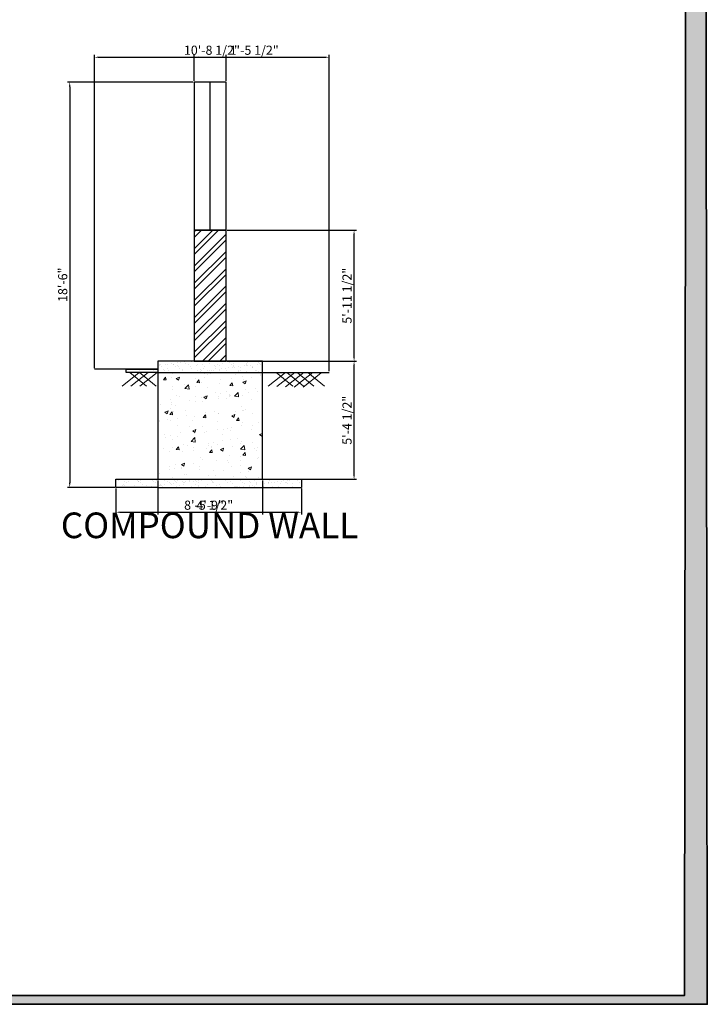
# Model space of a CAD drawing. Units: inches. Extents: x 1804 to 3296, y 909 to 2477.
# Tile 24 of 31: x 2920 to 3296, y 909 to 1449. Entities that reach past the tile are written whole.
import ezdxf

# ---------------------------------------------------------------- set-up
doc = ezdxf.new("R2010")
doc.units = ezdxf.units.IN
for name, color, linetype, lineweight in [('A-ANNO-DIMS', 2, 'Continuous', 18), ('A-ANNO-TTLB', 156, 'Continuous', 35), ('A-DETL', 7, 'Continuous', 30), ('A-DETL-PATT', 8, 'Continuous', 13), ('A-WALL-PATT', 10, 'Continuous', 13), ('C-GRAD-PATT', 8, 'Continuous', 13), ('TEXT', 190, 'Continuous', 18)]:
    doc.layers.add(name, color=color, linetype=linetype, lineweight=lineweight)
doc.styles.get("Standard").update_dxf_attribs({"font": 'arial.ttf'})
doc.dimstyles.new('ISO-25', dxfattribs={"dimtxt": 5, "dimasz": 2.5, "dimexe": 1.25, "dimexo": 0.625, "dimtad": 1, "dimdec": 0, "dimlunit": 4, "dimtxsty": 'Standard', "dimcen": 2.5, "dimadec": 0, "dimazin": 0, "dimtfac": 1, "dimtdec": 0, "dimtmove": 0, "dimatfit": 3, "dimfxl": 1, "dimarcsym": 0})

# ---------------------------------------------------------------- blocks, each defined once
blk = doc.blocks.new('*D94')
at = {"layer": 'A-ANNO-DIMS', "color": 0, "lineweight": -2, "transparency": 16777216}
for p, q in [((2972.46, 1191.87), (2972.46, 1177.65)), ((3074, 1191.87), (3074, 1177.65)), ((2974.96, 1178.9), (3071.5, 1178.9))]:
    blk.add_line(p, q, dxfattribs=at)
at = {"layer": 'A-ANNO-DIMS', "color": 0, "lineweight": 100, "transparency": 16777216}
for points in [[(2974.96, 1179.31), (2974.96, 1178.48), (2972.46, 1178.9)], [(3071.5, 1179.31), (3071.5, 1178.48), (3074, 1178.9)]]:
    blk.add_solid(points, dxfattribs=at)
at = {"layer": 'Defpoints', "color": 0, "lineweight": 100, "transparency": 16777216}
for p in [(2972.46, 1192.5), (3074, 1192.5), (3074, 1178.9)]:
    blk.add_point(p, dxfattribs=at)
at = {"layer": 'A-ANNO-DIMS', "color": 0, "transparency": 16777216, "insert": (3023.23, 1182.11), "char_height": 5, "attachment_point": 5}
blk.add_mtext('8\'-5 1/2"', dxfattribs=at)
blk = doc.blocks.new('*D95')
at = {"layer": 'A-ANNO-DIMS', "color": 0, "lineweight": -2, "transparency": 16777216}
for p, q in [((3014.75, 1414.4), (2945.94, 1414.4)), ((2947.19, 1411.9), (2947.19, 1195)), ((2971.84, 1192.5), (2945.94, 1192.5))]:
    blk.add_line(p, q, dxfattribs=at)
at = {"layer": 'A-ANNO-DIMS', "color": 0, "lineweight": 100, "transparency": 16777216}
for points in [[(2946.78, 1411.9), (2947.61, 1411.9), (2947.19, 1414.4)], [(2946.78, 1195), (2947.61, 1195), (2947.19, 1192.5)]]:
    blk.add_solid(points, dxfattribs=at)
at = {"layer": 'Defpoints', "color": 0, "lineweight": 100, "transparency": 16777216}
for p in [(3015.37, 1414.4), (2947.19, 1192.5), (2972.46, 1192.5)]:
    blk.add_point(p, dxfattribs=at)
at = {"layer": 'A-ANNO-DIMS', "color": 0, "transparency": 16777216, "insert": (2944.01, 1303.45), "char_height": 5, "attachment_point": 5, "rotation": 90}
blk.add_mtext('18\'-6"', dxfattribs=at)
blk = doc.blocks.new('*D96')
at = {"layer": 'A-ANNO-DIMS', "color": 0, "lineweight": -2, "transparency": 16777216}
for p, q in [((3015.37, 1415.02), (3015.37, 1429.25)), ((3032.82, 1415.02), (3032.82, 1429.25)), ((3017.87, 1428), (3030.32, 1428)), ((3032.82, 1428), (3061.04, 1428))]:
    blk.add_line(p, q, dxfattribs=at)
at = {"layer": 'A-ANNO-DIMS', "color": 0, "lineweight": 100, "transparency": 16777216}
for points in [[(3017.87, 1428.42), (3017.87, 1427.58), (3015.37, 1428)], [(3030.32, 1428.42), (3030.32, 1427.58), (3032.82, 1428)]]:
    blk.add_solid(points, dxfattribs=at)
at = {"layer": 'Defpoints', "color": 0, "lineweight": 100, "transparency": 16777216}
for p in [(3032.82, 1428), (3015.37, 1414.4), (3032.82, 1414.4)]:
    blk.add_point(p, dxfattribs=at)
at = {"layer": 'A-ANNO-DIMS', "color": 0, "transparency": 16777216, "insert": (3048.18, 1431.21), "char_height": 5, "attachment_point": 5}
blk.add_mtext('1\'-5 1/2"', dxfattribs=at)
blk = doc.blocks.new('*D97')
at = {"layer": 'A-ANNO-DIMS', "color": 0, "lineweight": -2, "transparency": 16777216}
for p, q in [((2995.47, 1196.29), (2995.47, 1177.65)), ((3052.66, 1196.29), (3052.66, 1177.65)), ((2997.97, 1178.9), (3050.16, 1178.9))]:
    blk.add_line(p, q, dxfattribs=at)
at = {"layer": 'A-ANNO-DIMS', "color": 0, "lineweight": 100, "transparency": 16777216}
for points in [[(2997.97, 1179.31), (2997.97, 1178.48), (2995.47, 1178.9)], [(3050.16, 1179.31), (3050.16, 1178.48), (3052.66, 1178.9)]]:
    blk.add_solid(points, dxfattribs=at)
at = {"layer": 'Defpoints', "color": 0, "lineweight": 100, "transparency": 16777216}
for p in [(2995.47, 1196.92), (3052.66, 1196.92), (3052.66, 1178.9)]:
    blk.add_point(p, dxfattribs=at)
at = {"layer": 'A-ANNO-DIMS', "color": 0, "transparency": 16777216, "insert": (3024.06, 1182.07), "char_height": 5, "attachment_point": 5}
blk.add_mtext('4\'-9"', dxfattribs=at)
blk = doc.blocks.new('*D98')
at = {"layer": 'A-ANNO-DIMS', "color": 0, "lineweight": -2, "transparency": 16777216}
for p, q in [((3053.28, 1261.58), (3104.08, 1261.58)), ((3102.83, 1199.42), (3102.83, 1259.08)), ((3053.28, 1196.92), (3104.08, 1196.92))]:
    blk.add_line(p, q, dxfattribs=at)
at = {"layer": 'A-ANNO-DIMS', "color": 0, "lineweight": 100, "transparency": 16777216}
for points in [[(3102.41, 1259.08), (3103.24, 1259.08), (3102.83, 1261.58)], [(3102.41, 1199.42), (3103.24, 1199.42), (3102.83, 1196.92)]]:
    blk.add_solid(points, dxfattribs=at)
at = {"layer": 'Defpoints', "color": 0, "lineweight": 100, "transparency": 16777216}
for p in [(3052.66, 1261.58), (3102.83, 1261.58), (3052.66, 1196.92)]:
    blk.add_point(p, dxfattribs=at)
at = {"layer": 'A-ANNO-DIMS', "color": 0, "transparency": 16777216, "insert": (3099.62, 1229.25), "char_height": 5, "attachment_point": 5, "rotation": 90}
blk.add_mtext('5\'-4 1/2"', dxfattribs=at)
blk = doc.blocks.new('*D99')
at = {"layer": 'A-ANNO-DIMS', "color": 0, "lineweight": -2, "transparency": 16777216}
for p, q in [((3033.45, 1333.28), (3104.08, 1333.28)), ((3102.83, 1264.08), (3102.83, 1330.78)), ((3033.45, 1261.58), (3104.08, 1261.58))]:
    blk.add_line(p, q, dxfattribs=at)
at = {"layer": 'A-ANNO-DIMS', "color": 0, "lineweight": 100, "transparency": 16777216}
for points in [[(3102.41, 1330.78), (3103.24, 1330.78), (3102.83, 1333.28)], [(3102.41, 1264.08), (3103.24, 1264.08), (3102.83, 1261.58)]]:
    blk.add_solid(points, dxfattribs=at)
at = {"layer": 'Defpoints', "color": 0, "lineweight": 100, "transparency": 16777216}
for p in [(3032.82, 1333.28), (3102.83, 1333.28), (3032.82, 1261.58)]:
    blk.add_point(p, dxfattribs=at)
at = {"layer": 'A-ANNO-DIMS', "color": 0, "transparency": 16777216, "insert": (3099.62, 1297.43), "char_height": 5, "attachment_point": 5, "rotation": 90}
blk.add_mtext('5\'-11 1/2"', dxfattribs=at)
blk = doc.blocks.new('*D100')
at = {"layer": 'A-ANNO-DIMS', "color": 0, "lineweight": -2, "transparency": 16777216}
for p, q in [((2960.79, 1257.86), (2960.79, 1429.25)), ((3089.23, 1256.09), (3089.23, 1429.25)), ((2963.29, 1428), (3086.73, 1428))]:
    blk.add_line(p, q, dxfattribs=at)
at = {"layer": 'A-ANNO-DIMS', "color": 0, "lineweight": 100, "transparency": 16777216}
for points in [[(2963.29, 1428.42), (2963.29, 1427.58), (2960.79, 1428)], [(3086.73, 1428.42), (3086.73, 1427.58), (3089.23, 1428)]]:
    blk.add_solid(points, dxfattribs=at)
at = {"layer": 'Defpoints', "color": 0, "lineweight": 100, "transparency": 16777216}
for p in [(3089.23, 1428), (2960.79, 1257.24), (3089.23, 1255.47)]:
    blk.add_point(p, dxfattribs=at)
at = {"layer": 'A-ANNO-DIMS', "color": 0, "transparency": 16777216, "insert": (3025.01, 1431.21), "char_height": 5, "attachment_point": 5}
blk.add_mtext('10\'-8 1/2"', dxfattribs=at)

msp = doc.modelspace()

# ---------------------------------------------------------------- hatches: boundary and pattern name
at = {"layer": 'A-ANNO-TTLB'}
h = msp.add_hatch(color=256, dxfattribs=at)
h.dxf.hatch_style = 1
h.paths.add_polyline_path([(3294.53, 2476.54), (1803.79, 2476.54), (1805.43, 909.47), (3296.17, 909.47)])
h.paths.add_polyline_path([(1811, 914.33), (1812.79, 2467.54), (3285.53, 2467.54), (3283.74, 914.33)], flags=16)
h.paths.add_polyline_path([(1925.58, 1062.77), (1925.58, 1138.07), (1925.58, 1539.88), (1925.58, 1793.38), (1925.58, 1830.04), (2325.54, 1830.04), (2325.54, 1793.38), (2325.54, 1586.42), (2325.54, 1138.07), (2325.54, 1062.77)], flags=0)
h.paths.add_polyline_path([(1997.22, 1029.4), (2008.85, 1037.96), (2008.85, 1020.84)], flags=0)
h.paths.add_polyline_path([(1934.58, 1138.07), (1934.58, 1147.07), (2078.77, 1147.07), (2078.77, 1138.07), (2060.94, 1138.07)], flags=0)
h.paths.add_polyline_path([(1944.35, 1138.07), (1944.35, 1147.07), (2056.05, 1147.07), (2056.05, 1138.07)], flags=0)
h.paths.add_polyline_path([(2222.24, 1037.96), (2233.87, 1029.4), (2222.24, 1020.84)], flags=0)
h.paths.add_polyline_path([(2061.94, 1139.07), (2061.94, 1146.07), (2077.77, 1146.07), (2077.77, 1139.07)], flags=0)
h.paths.add_polyline_path([(2149.58, 1138.07), (2149.58, 1269.44), (2158.58, 1269.44), (2158.58, 1326.69), (2149.58, 1326.69), (2149.58, 1340.94), (2139.6, 1340.94), (2139.6, 1434.25), (2149.58, 1434.25), (2149.58, 1447.36), (2158.58, 1447.36), (2158.58, 1423.87), (2158.58, 1408.06), (2198.46, 1408.06), (2198.46, 1412.56), (2282.65, 1412.56), (2282.65, 1465.94), (2316.54, 1465.94), (2316.54, 1590.92), (2192.86, 1590.92), (2192.86, 1595.3), (2291.17, 1595.3), (2291.17, 1590.92), (2316.54, 1590.92), (2316.54, 1784.38), (2300.24, 1784.38), (2300.24, 1757.47), (2268, 1757.47), (2268, 1681.04), (2180.87, 1681.04), (2180.87, 1757.47), (2148.63, 1757.47), (2148.63, 1784.38), (2119.08, 1784.38), (2119.08, 1585.58), (2114.58, 1585.58), (2114.58, 1784.38), (2064.11, 1784.38), (2046.28, 1784.38), (2046.28, 1760.38), (1958.58, 1760.38), (1958.58, 1664.38), (1934.58, 1664.38), (1934.58, 1784.38), (1934.58, 1793.38), (2046.28, 1793.38), (2064.11, 1793.38), (2119.08, 1793.38), (2230.78, 1793.38), (2230.78, 1784.38), (2268, 1784.38), (2300.24, 1784.38), (2316.54, 1784.38), (2316.54, 1590.92), (2316.54, 1373.73), (2316.54, 1138.07)], flags=0)
h.paths.add_polyline_path([(2209.19, 1166.63), (2209.19, 1175.63), (2158.58, 1175.63), (2209.19, 1223.63), (2209.19, 1231.63), (2183.88, 1231.63), (2183.88, 1301.66), (2242.59, 1301.66), (2242.59, 1326.69), (2316.54, 1326.69), (2272.59, 1271.63), (2272.59, 1223.63), (2316.54, 1175.63), (2272.59, 1175.63), (2272.59, 1166.63)], flags=0)
h.paths.add_polyline_path([(1947.77, 1345.22), (1947.77, 1457.48), (1991.2, 1457.48), (1991.2, 1451.7), (1991.2, 1352.18), (1991.2, 1345.22)], flags=0)
h.paths.add_polyline_path([(2209.19, 1271.63), (2262.59, 1271.63), (2262.59, 1311.85), (2272.59, 1301.66), (2272.59, 1271.63), (2269.92, 1269.63), (2270.59, 1269.63), (2270.59, 1225.63), (2211.19, 1225.63), (2211.19, 1269.63), (2211.86, 1269.63)], flags=0)
h.paths.add_polyline_path([(2000.34, 1378.21), (2000.34, 1429.71), (2025.22, 1429.71), (2025.22, 1378.21)], flags=0)
h.paths.add_polyline_path([(2001.34, 1379.21), (2001.34, 1428.71), (2024.22, 1428.71), (2024.22, 1379.21)], flags=0)
h.paths.add_polyline_path([(2012.34, 1390.21), (2012.34, 1417.71), (2013.22, 1417.71), (2013.22, 1390.21)], flags=0)
h.paths.add_polyline_path([(2237.56, 1331.19), (2237.56, 1340.18), (2238.62, 1340.18), (2238.62, 1386.84), (2241.04, 1386.84), (2242.06, 1386.84), (2242.06, 1408.06), (2316.54, 1331.19)], flags=0)
h.paths.add_polyline_path([(1953.73, 1464.35), (1953.73, 1498.59), (1981.74, 1498.59), (1981.74, 1464.35)], flags=0)
h.paths.add_polyline_path([(1987.63, 1462.08), (1987.63, 1500.95), (2104.07, 1500.95), (2104.07, 1462.08), (2099.27, 1462.08), (1993.6, 1462.08)], flags=0)
h.paths.add_polyline_path([(1956.06, 1481.47, -1), (1979.41, 1481.47, -1)], flags=0)
edge = h.paths.add_edge_path(flags=0)
edge.add_ellipse((2299.53, 1438.37), major_axis=(0.31, 21.36), ratio=0.670333, start_angle=0, end_angle=360)
h.paths.add_polyline_path([(2297.39, 1438.37, -1), (2301.67, 1438.37, -1)], flags=0)
h.paths.add_polyline_path([(2591.54, 1163.23), (2591.54, 1179.38), (2591.54, 1379.68), (2591.54, 1395.84), (2734.5, 1395.84), (2734.5, 1379.68), (2734.5, 1179.38), (2734.5, 1163.23)], flags=0)
h.paths.add_polyline_path([(2592.54, 1164.23), (2592.54, 1166.23), (2733.5, 1166.23), (2733.5, 1164.23)], flags=0)
h.paths.add_polyline_path([(2592.54, 1180.38), (2592.54, 1378.68), (2733.5, 1378.68), (2733.5, 1180.38)], flags=0)
h.paths.add_polyline_path([(2593.54, 1181.38), (2593.54, 1377.68), (2732.5, 1377.68), (2732.5, 1181.38)], flags=0)
h.paths.add_polyline_path([(2594.54, 1182.38), (2594.54, 1376.68), (2731.5, 1376.68), (2731.5, 1182.38)], flags=0)
h.paths.add_polyline_path([(1936.95, 1697.46), (1936.95, 1736.46), (1955.41, 1736.46), (1955.41, 1697.46)], flags=0)
h.paths.add_polyline_path([(1938.48, 1718.36), (1938.48, 1734.92), (1953.65, 1734.92), (1953.65, 1718.36)], flags=0)
h.paths.add_polyline_path([(1944.75, 1726.64, -1), (1947.37, 1726.64, -1)], flags=0)
h.paths.add_polyline_path([(2592.54, 1394.84), (2733.5, 1394.84), (2733.5, 1392.84), (2592.54, 1392.84)], flags=0)
h.paths.add_polyline_path([(1976.61, 1762.5), (1976.61, 1781.44), (2012.79, 1781.44), (2012.79, 1762.5)], flags=0)
h.paths.add_polyline_path([(1979.57, 1771.97, -1), (1991.39, 1771.97, -1)], flags=0)
h.paths.add_polyline_path([(1995.36, 1771.97, -1), (2007.18, 1771.97, -1)], flags=0)
h.paths.add_polyline_path([(2251.51, 1744.53), (2268, 1730.05), (2251.51, 1730.05)], flags=0)
h.paths.add_polyline_path([(2047.28, 1785.38), (2047.28, 1792.38), (2063.11, 1792.38), (2063.11, 1785.38)], flags=0)
h.paths.add_polyline_path([(2155.08, 1770.92, -1), (2174.42, 1770.92, -1)], flags=0)
h.paths.add_polyline_path([(2188.59, 1758.27), (2188.59, 1772.81), (2222.3, 1772.81), (2222.3, 1758.27)], flags=0)
h.paths.add_polyline_path([(2223.97, 1758.27), (2223.97, 1772.81), (2257.68, 1772.81), (2257.68, 1758.27)], flags=0)
h.paths.add_polyline_path([(2274.45, 1770.92, -1), (2293.8, 1770.92, -1)], flags=0)
h.paths.add_polyline_path([(2591.54, 1582.09), (2591.54, 1782.39), (2734.5, 1782.39), (2734.5, 1582.09)], flags=0)
h.paths.add_polyline_path([(2592.54, 1583.09), (2592.54, 1781.39), (2733.5, 1781.39), (2733.5, 1583.09)], flags=0)
h.paths.add_polyline_path([(2593.54, 1584.09), (2593.54, 1780.39), (2732.5, 1780.39), (2732.5, 1584.09)], flags=0)
h.paths.add_polyline_path([(2594.54, 1585.09), (2594.54, 1779.39), (2731.5, 1779.39), (2731.5, 1585.09)], flags=0)
h.paths.add_polyline_path([(1922.17, 1978.79), (1922.17, 2295.08), (1922.17, 2296.08), (2115.67, 2296.08), (2115.67, 2384.31), (2115.67, 2385.31), (2322.12, 2385.31), (2323.12, 2385.31), (2323.12, 1979.79), (2323.12, 1978.79), (1923.17, 1978.79)], flags=0)
h.paths.add_polyline_path([(1922.17, 1978.79), (1922.17, 2051.31), (1922.17, 2214.86), (1922.17, 2296.08), (2115.67, 2296.08), (2115.67, 2385.31), (2323.12, 2385.31), (2323.12, 2280.42), (2323.12, 1978.79), (2115.67, 1978.79)], flags=0)
h.paths.add_polyline_path([(1923.17, 1979.79), (1923.17, 2050.31), (2115.67, 2050.31), (2115.67, 2051.31), (1923.17, 2051.31), (1923.17, 2213.86), (1923.17, 2214.86), (1923.17, 2295.08), (1990.02, 2295.08), (1990.02, 2214.86), (1991.02, 2214.86), (1991.02, 2295.08), (2115.67, 2295.08), (2115.67, 1979.79), (2116.67, 1979.79), (2116.67, 2304.18), (2116.67, 2384.31), (2322.12, 2384.31), (2322.12, 2280.42), (2322.12, 1979.79), (2115.67, 1979.79)], flags=0)
h.paths.add_polyline_path([(2972.46, 1192.5), (2972.46, 1196.92), (2995.47, 1196.92), (2995.47, 1255.47), (2995.09, 1255.47), (2987.42, 1249.39), (2980.08, 1255.47), (2978.05, 1255.47), (2978.05, 1257.24), (2995.47, 1257.24), (2995.47, 1261.58), (3015.37, 1261.58), (3015.37, 1333.28), (3015.37, 1414.4), (3032.82, 1414.4), (3032.82, 1333.28), (3032.82, 1261.58), (3052.66, 1261.58), (3052.66, 1255.47), (3079.86, 1255.47), (3078.72, 1254.57), (3081.47, 1252.29), (3078.56, 1249.99), (3075.81, 1252.26), (3072.57, 1249.69), (3070.36, 1251.52), (3067.67, 1249.39), (3060.34, 1255.47), (3052.66, 1255.47), (3052.66, 1196.92), (3054.58, 1196.92), (3074, 1196.92), (3074, 1192.5), (3052.66, 1192.5), (2995.47, 1192.5)], flags=0)
h.paths.add_polyline_path([(2490.75, 1979.27), (2490.75, 1980.27), (2596.87, 1980.27), (2596.87, 2051.8), (2596.87, 2052.8), (2596.87, 2216.35), (2596.87, 2297.57), (2717.32, 2297.57), (2710.57, 2305.62), (2724.07, 2305.62), (2717.32, 2297.57), (2782.37, 2297.57), (2782.37, 2395.8), (3006.82, 2395.8), (3006.82, 1981.27), (3093.73, 1981.27), (3093.73, 1980.27), (3047.51, 1980.27), (3046.37, 1979.37), (3049.11, 1977.1), (3046.2, 1974.79), (3043.46, 1977.07), (3040.21, 1974.49), (3038, 1976.32), (3035.32, 1974.2), (3027.98, 1980.27), (2871.83, 1980.27), (2871.83, 1981.27), (2791.37, 1981.27), (2791.37, 2050.8), (2597.87, 2050.8), (2597.87, 1980.27), (2597.87, 1979.27), (2546.27, 1979.27), (2545.12, 1978.37), (2547.87, 1976.1), (2544.96, 1973.79), (2542.22, 1976.07), (2538.97, 1973.49), (2536.76, 1975.32), (2534.07, 1973.2), (2526.74, 1979.27)], flags=0)
h.paths.add_polyline_path([(2597.87, 2051.8), (2606.87, 2051.8), (2606.87, 2258.39), (2597.87, 2258.39), (2597.87, 2296.57), (2606.87, 2296.57), (2606.87, 2262.39), (2782.37, 2262.39), (2782.37, 2296.57), (2790.37, 2296.57), (2790.37, 2262.39), (2791.37, 2262.39), (2791.37, 2305.67), (2791.37, 2385.8), (2996.82, 2385.8), (2996.82, 2339.85), (3006.82, 2339.85), (3006.82, 2250.12), (2997.82, 2250.12), (2997.82, 1981.27), (2996.82, 1981.27), (2872.83, 1981.27), (2872.83, 1991.8), (2871.83, 1991.8), (2871.83, 2050.8), (2790.37, 2050.8), (2597.87, 2050.8)], flags=0)
h.paths.add_polyline_path([(2179.93, 2153.92), (2179.93, 2353.97), (2259.98, 2353.97), (2259.98, 2153.92)], flags=0)
h.paths.add_polyline_path([(2180.93, 2154.92), (2180.93, 2352.97), (2258.98, 2352.97), (2258.98, 2154.92)], flags=0)
h.paths.add_polyline_path([(2960.87, 1608.49), (2960.87, 1753.62), (3070.9, 1753.62), (3070.9, 1608.49)], flags=0)
h.paths.add_polyline_path([(2961.87, 1609.49), (2961.87, 1752.62), (3069.9, 1752.62), (3069.9, 1609.49)], flags=0)
h.paths.add_polyline_path([(2962.87, 1610.49), (2962.87, 1751.62), (3068.9, 1751.62), (3068.9, 1610.49)], flags=0)
h.paths.add_polyline_path([(2963.87, 1611.49), (2963.87, 1750.62), (3067.9, 1750.62), (3067.9, 1611.49)], flags=0)
h.paths.add_polyline_path([(2782.37, 2051.8), (2782.37, 2216.32), (2791.37, 2216.32), (2791.37, 2051.8), (2872.83, 2051.8), (2872.83, 2068.56), (2884.67, 2068.56), (2884.67, 2085.33), (2896.51, 2085.33), (2896.51, 2102.09), (2908.36, 2102.09), (2908.36, 2118.85), (2920.2, 2118.85), (2920.2, 2135.62), (2932.05, 2135.62), (2932.05, 2145.3), (2925.08, 2145.3), (2925.08, 2203.2), (2996.82, 2203.2), (2996.82, 2145.3), (2953.82, 2145.3), (2872.83, 2051.8), (2790.37, 2051.8)], flags=0)
h.paths.add_polyline_path([(2717.32, 2238.65), (2710.57, 2246.7), (2724.07, 2246.7)], flags=0)
h.paths.add_polyline_path([(2003.09, 1122.79), (2017.16, 1122.79), (2017.16, 1138.74), (2003.09, 1138.74)], flags=8)
h.paths.add_polyline_path([(2174.76, 1792.72), (2188.83, 1792.72), (2188.83, 1808.66), (2174.76, 1808.66)], flags=8)
h.paths.add_polyline_path([(1987.95, 1792.51), (2002.02, 1792.51), (2002.02, 1808.45), (1987.95, 1808.45)], flags=8)
h.paths.add_polyline_path([(2148.79, 1289.26), (2160.46, 1289.26), (2160.46, 1305.2), (2148.79, 1305.2)], flags=8)
h.paths.add_polyline_path([(2115.36, 1133.57), (2127.04, 1133.57), (2127.04, 1149.51), (2115.36, 1149.51)], flags=8)
h.paths.add_polyline_path([(2237.58, 1421.48), (2249.25, 1421.48), (2249.25, 1437.43), (2237.58, 1437.43)], flags=8)
h.paths.add_polyline_path([(2134.99, 1584.32), (2146.66, 1584.32), (2146.66, 1600.26), (2134.99, 1600.26)], flags=8)
h.paths.add_polyline_path([(2101.95, 1557.31), (2113.62, 1557.31), (2113.62, 1573.25), (2101.95, 1573.25)], flags=8)
h.paths.add_polyline_path([(2937.85, 1156.77), (3120.41, 1156.77), (3120.41, 1185.72), (2937.85, 1185.72)], flags=8)
h.paths.add_polyline_path([(2980.71, 1786.71), (3050.06, 1786.71), (3050.06, 1802.66), (2980.71, 1802.66)], flags=8)
h.paths.add_polyline_path([(2869.28, 1661.96), (2938.62, 1661.96), (2938.62, 1690.8), (2869.28, 1690.8)], flags=8)
h.paths.add_polyline_path([(3092.27, 1674.86), (3161.62, 1674.86), (3161.62, 1690.8), (3092.27, 1690.8)], flags=8)
h.paths.add_polyline_path([(2980.71, 1674.86), (3050.06, 1674.86), (3050.06, 1690.8), (2980.71, 1690.8)], flags=8)
h.paths.add_polyline_path([(2649.07, 1678.23), (2674.53, 1678.23), (2674.53, 1714.76), (2649.07, 1714.76)], flags=8)
h.paths.add_polyline_path([(2530.84, 1981.63), (2549.13, 1981.63), (2549.13, 1997.57), (2530.84, 1997.57)], flags=8)
h.paths.add_polyline_path([(3031.29, 1981.77), (3049.58, 1981.77), (3049.58, 1997.71), (3031.29, 1997.71)], flags=8)
h.paths.add_polyline_path([(2715.38, 1911.9), (2851.54, 1911.9), (2851.54, 1940.85), (2715.38, 1940.85)], flags=8)
h.paths.add_polyline_path([(2015.23, 1927.36), (2205.42, 1927.36), (2205.42, 1956.3), (2015.23, 1956.3)], flags=8)
h.paths.add_polyline_path([(2671.84, 2057.84), (2702.75, 2057.84), (2702.75, 2073.79), (2671.84, 2073.79)], flags=8)
h.paths.add_polyline_path([(2678.5, 2316.52), (2765.26, 2316.52), (2765.26, 2332.46), (2678.5, 2332.46)], flags=8)
h.paths.add_polyline_path([(2678.48, 2271.96), (2736.41, 2271.96), (2736.41, 2287.9), (2678.48, 2287.9)], flags=8)
h.paths.add_polyline_path([(2019.2, 972.79), (2243.21, 972.79), (2243.21, 1001.74), (2019.2, 1001.74)], flags=8)
h.paths.add_polyline_path([(2097.06, 1021.56), (2132.16, 1021.56), (2132.16, 1037.51), (2097.06, 1037.51)], flags=8)
h.paths.add_polyline_path([(2182.47, 1360.48), (2207.35, 1360.48), (2207.35, 1376.42), (2182.47, 1376.42)], flags=8)
h.paths.add_polyline_path([(2261.12, 1361.77), (2295.01, 1361.77), (2295.01, 1377.71), (2261.12, 1377.71)], flags=8)
h.paths.add_polyline_path([(2245.75, 1511.51), (2278.44, 1511.51), (2278.44, 1527.46), (2245.75, 1527.46)], flags=8)
h.paths.add_polyline_path([(1991.16, 1296.29), (2060.51, 1296.29), (2060.51, 1312.23), (1991.16, 1312.23)], flags=8)
h.paths.add_polyline_path([(2187, 1651.35), (2246.71, 1651.35), (2246.71, 1667.29), (2187, 1667.29)], flags=8)
h.paths.add_polyline_path([(1976.49, 1684.81), (2068.63, 1684.81), (2068.63, 1700.76), (1976.49, 1700.76)], flags=8)
at = {"layer": 'A-DETL-PATT'}
h = msp.add_hatch(dxfattribs=at)
h.set_pattern_fill('ANSI32', color=256, scale=0.7)
h.set_pattern_definition([(45, (64.579, 248.7134), (-4.714634, 4.714634), []), (45, (67.722, 248.7134), (-4.714634, 4.714634), [])])
h.paths.add_polyline_path([(3032.82, 1333.28), (3015.37, 1333.28), (3015.37, 1261.58), (3032.82, 1261.58)])
h = msp.add_hatch(dxfattribs=at)
h.set_pattern_fill('AR-SAND', color=256, scale=0.1)
h.set_pattern_definition([(37.5, (64.579, 248.7134), (-0.160003, 4.8941324), [0, -3.8608, 0, -4.318, 0, -4.1275]), (7.5, (64.579, 248.7134), (4.495233, 7.168251), [0, -2.0828, 0, -3.4798, 0, -1.3335]), (327.5, (61.4548, 248.7134), (7.9099237, 0.014372), [0, -1.27, 0, -4.572, 0, -5.969]), (317.5, (61.455, 248.7134), (7.635565, 2.229293), [0, -0.635, 0, -2.9972, 0, -3.429])])
h.paths.add_polyline_path([(3052.66, 1261.58), (2995.47, 1261.58), (2995.47, 1255.47), (3052.66, 1255.47)])
h.paths.add_polyline_path([(3074, 1196.92), (3052.66, 1196.92), (2995.47, 1196.92), (2972.46, 1196.92), (2972.46, 1192.5), (2995.47, 1192.5), (3052.66, 1192.5), (3074, 1192.5)])
h.paths.add_polyline_path([(2995.47, 1257.24), (2978.05, 1257.24), (2978.05, 1255.47), (2995.47, 1255.47)])
h = msp.add_hatch(dxfattribs=at)
h.set_pattern_fill('AR-SAND', color=256, scale=0.4)
h.set_pattern_definition([(37.5, (64.579, 248.713), (-0.64001, 19.57653), [0, -15.4432, 0, -17.272, 0, -16.51]), (7.5, (64.58, 248.713), (17.98093, 28.673), [0, -8.3312, 0, -13.9192, 0, -5.334]), (327.5, (52.082, 248.713), (31.639695, 0.05749), [0, -5.08, 0, -18.288, 0, -23.876]), (317.5, (52.082, 248.713), (30.54226, 8.91717), [0, -2.54, 0, -11.9888, 0, -13.716])])
h.paths.add_polyline_path([(2995.47, 1196.92), (3052.66, 1196.92), (3052.66, 1255.47), (2995.47, 1255.47)])
h = msp.add_hatch(dxfattribs=at)
h.set_pattern_fill('AR-CONC', color=256, scale=0.1)
h.set_pattern_definition([(50, (64.579, 248.713), (18.21847, -1.59391), [1.905, -20.955]), (355, (64.579, 248.713), (-3.52434, 19.10568), [1.524, -16.76406]), (100.45144, (66.097, 248.58), (14.69412, 17.51178), [1.619, -17.80902]), (46.1842, (64.58, 253.793), (27.1079, -4.20423), [2.8575, -31.4325]), (96.6356, (66.838, 253.443), (23.74041, 24.74261), [2.4285, -26.71356]), (351.1842, (64.58, 253.793), (23.74041, 24.7426), [2.286, -25.14597]), (21, (67.119, 252.523), (15.16144, -10.22652), [1.905, -20.955]), (326, (67.119, 252.523), (6.1802, 18.4188), [1.524, -16.764]), (71.45144, (68.382, 251.671), (21.34164, 8.19228), [1.619, -17.80899]), (37.5, (64.579, 248.7134), (0.30886, 8.455504), [0, -16.5608, 0, -17.018, 0, -16.8275]), (7.5, (64.579, 248.713), (6.681966, 10.018057), [0, -9.7028, 0, -16.1798, 0, -6.4135]), (327.5, (58.915, 248.7134), (13.55906, -0.572874), [0, -6.35, 0, -19.812, 0, -26.289]), (317.5, (56.375, 248.713), (14.81292, 2.54265), [0, -8.255, 0, -13.1572, 0, -18.669])])
h.paths.add_polyline_path([(2995.47, 1255.47), (2995.47, 1196.92), (3052.66, 1196.92), (3052.66, 1255.47)])
at = {"layer": 'A-WALL-PATT'}
h = msp.add_hatch(color=256, dxfattribs=at)
h.dxf.hatch_style = 1
h.paths.add_polyline_path([(2119.08, 1544.38), (1925.58, 1544.38), (1925.58, 1539.88), (2119.08, 1539.88)])
h.paths.add_polyline_path([(2119.08, 1545.58), (2114.58, 1545.58), (2114.58, 1544.38), (2119.08, 1544.38)])
h.paths.add_polyline_path([(1965.87, 1658.79), (1965.87, 1679.09), (1955.57, 1679.09), (1955.57, 1658.79)], flags=9)
h.paths.add_polyline_path([(2293.18, 1677.29), (2293.18, 1697.58), (2282.88, 1697.58), (2282.88, 1677.29)], flags=9)
h.paths.add_polyline_path([(2271.13, 1545.23), (2287.53, 1545.23), (2287.53, 1555.53), (2271.13, 1555.53)], flags=9)
h.paths.add_polyline_path([(2303.26, 1488.52), (2303.26, 1508.82), (2292.95, 1508.82), (2292.95, 1488.52)], flags=9)
h.paths.add_polyline_path([(2271.13, 1393.15), (2287.53, 1393.15), (2287.53, 1403.45), (2271.13, 1403.45)], flags=9)
h.paths.add_polyline_path([(2306.48, 1361.45), (2306.48, 1377.86), (2296.18, 1377.86), (2296.18, 1361.45)], flags=9)
h.paths.add_polyline_path([(2174.54, 1361.45), (2174.54, 1377.86), (2164.23, 1377.86), (2164.23, 1361.45)], flags=9)
h.paths.add_polyline_path([(1968.21, 1333.34), (1968.21, 1353.64), (1957.91, 1353.64), (1957.91, 1333.34)], flags=9)
h.paths.add_polyline_path([(2003.09, 1122.79), (2017.16, 1122.79), (2017.16, 1138.74), (2003.09, 1138.74)], flags=9)
h.paths.add_polyline_path([(2174.76, 1792.72), (2188.83, 1792.72), (2188.83, 1808.66), (2174.76, 1808.66)], flags=9)
h.paths.add_polyline_path([(1987.95, 1792.51), (2002.02, 1792.51), (2002.02, 1808.45), (1987.95, 1808.45)], flags=9)
h.paths.add_polyline_path([(2148.79, 1289.26), (2160.46, 1289.26), (2160.46, 1305.2), (2148.79, 1305.2)], flags=9)
h.paths.add_polyline_path([(2115.36, 1133.57), (2127.04, 1133.57), (2127.04, 1149.51), (2115.36, 1149.51)], flags=9)
h.paths.add_polyline_path([(2237.58, 1421.48), (2249.25, 1421.48), (2249.25, 1437.43), (2237.58, 1437.43)], flags=9)
h.paths.add_polyline_path([(2134.99, 1584.32), (2146.66, 1584.32), (2146.66, 1600.26), (2134.99, 1600.26)], flags=9)
h.paths.add_polyline_path([(2101.95, 1557.31), (2113.62, 1557.31), (2113.62, 1573.25), (2101.95, 1573.25)], flags=9)
h.paths.add_polyline_path([(2937.85, 1156.77), (3120.41, 1156.77), (3120.41, 1185.72), (2937.85, 1185.72)], flags=9)
h.paths.add_polyline_path([(2980.71, 1786.71), (3050.06, 1786.71), (3050.06, 1802.66), (2980.71, 1802.66)], flags=9)
h.paths.add_polyline_path([(2869.28, 1661.96), (2938.62, 1661.96), (2938.62, 1690.8), (2869.28, 1690.8)], flags=9)
h.paths.add_polyline_path([(3092.27, 1674.86), (3161.62, 1674.86), (3161.62, 1690.8), (3092.27, 1690.8)], flags=9)
h.paths.add_polyline_path([(2980.71, 1674.86), (3050.06, 1674.86), (3050.06, 1690.8), (2980.71, 1690.8)], flags=9)
h.paths.add_polyline_path([(2649.07, 1678.23), (2674.53, 1678.23), (2674.53, 1714.76), (2649.07, 1714.76)], flags=9)
h.paths.add_polyline_path([(2530.84, 1981.63), (2549.13, 1981.63), (2549.13, 1997.57), (2530.84, 1997.57)], flags=9)
h.paths.add_polyline_path([(3031.29, 1981.77), (3049.58, 1981.77), (3049.58, 1997.71), (3031.29, 1997.71)], flags=9)
h.paths.add_polyline_path([(2715.38, 1911.9), (2851.54, 1911.9), (2851.54, 1940.85), (2715.38, 1940.85)], flags=9)
h.paths.add_polyline_path([(2015.23, 1927.36), (2205.42, 1927.36), (2205.42, 1956.3), (2015.23, 1956.3)], flags=9)
h.paths.add_polyline_path([(2671.84, 2057.84), (2702.75, 2057.84), (2702.75, 2073.79), (2671.84, 2073.79)], flags=9)
h.paths.add_polyline_path([(2678.5, 2316.52), (2765.26, 2316.52), (2765.26, 2332.46), (2678.5, 2332.46)], flags=9)
h.paths.add_polyline_path([(2678.48, 2271.96), (2736.41, 2271.96), (2736.41, 2287.9), (2678.48, 2287.9)], flags=9)
h.paths.add_polyline_path([(2019.2, 972.79), (2243.21, 972.79), (2243.21, 1001.74), (2019.2, 1001.74)], flags=9)
h.paths.add_polyline_path([(2097.06, 1021.56), (2132.16, 1021.56), (2132.16, 1037.51), (2097.06, 1037.51)], flags=9)
h.paths.add_polyline_path([(2182.47, 1360.48), (2207.35, 1360.48), (2207.35, 1376.42), (2182.47, 1376.42)], flags=9)
h.paths.add_polyline_path([(2261.12, 1361.77), (2295.01, 1361.77), (2295.01, 1377.71), (2261.12, 1377.71)], flags=9)
h.paths.add_polyline_path([(2245.75, 1511.51), (2278.44, 1511.51), (2278.44, 1527.46), (2245.75, 1527.46)], flags=9)
h.paths.add_polyline_path([(1991.16, 1296.29), (2060.51, 1296.29), (2060.51, 1312.23), (1991.16, 1312.23)], flags=9)
h.paths.add_polyline_path([(2187, 1651.35), (2246.71, 1651.35), (2246.71, 1667.29), (2187, 1667.29)], flags=9)
h.paths.add_polyline_path([(1976.49, 1684.81), (2068.63, 1684.81), (2068.63, 1700.76), (1976.49, 1700.76)], flags=9)
h = msp.add_hatch(color=256, dxfattribs=at)
h.dxf.hatch_style = 1
h.paths.add_polyline_path([(2149.58, 1147.07), (2141.21, 1147.07), (2141.21, 1144.07), (2141.21, 1138.07), (2149.58, 1138.07)])
h.paths.add_polyline_path([(2101.21, 1144.07, -0.01877), (2101.32, 1147.07), (2078.77, 1147.07), (2078.77, 1138.07), (2101.21, 1138.07)])
h.paths.add_polyline_path([(2060.94, 1147.07), (2056.05, 1147.07), (2056.05, 1138.07), (2060.94, 1138.07)])
h.paths.add_polyline_path([(1944.35, 1147.07), (1934.58, 1147.07), (1934.58, 1138.07), (1944.35, 1138.07)])
h.paths.add_polyline_path([(2158.58, 1269.44), (2149.58, 1269.44), (2149.58, 1138.07), (2158.58, 1138.07)])
h.paths.add_polyline_path([(2003.09, 1122.79), (2017.16, 1122.79), (2017.16, 1138.74), (2003.09, 1138.74)], flags=9)
h.paths.add_polyline_path([(2174.76, 1792.72), (2188.83, 1792.72), (2188.83, 1808.66), (2174.76, 1808.66)], flags=9)
h.paths.add_polyline_path([(1987.95, 1792.51), (2002.02, 1792.51), (2002.02, 1808.45), (1987.95, 1808.45)], flags=9)
h.paths.add_polyline_path([(2148.79, 1289.26), (2160.46, 1289.26), (2160.46, 1305.2), (2148.79, 1305.2)], flags=9)
h.paths.add_polyline_path([(2115.36, 1133.57), (2127.04, 1133.57), (2127.04, 1149.51), (2115.36, 1149.51)], flags=9)
h.paths.add_polyline_path([(2237.58, 1421.48), (2249.25, 1421.48), (2249.25, 1437.43), (2237.58, 1437.43)], flags=9)
h.paths.add_polyline_path([(2134.99, 1584.32), (2146.66, 1584.32), (2146.66, 1600.26), (2134.99, 1600.26)], flags=9)
h.paths.add_polyline_path([(2101.95, 1557.31), (2113.62, 1557.31), (2113.62, 1573.25), (2101.95, 1573.25)], flags=9)
h.paths.add_polyline_path([(2937.85, 1156.77), (3120.41, 1156.77), (3120.41, 1185.72), (2937.85, 1185.72)], flags=9)
h.paths.add_polyline_path([(2980.71, 1786.71), (3050.06, 1786.71), (3050.06, 1802.66), (2980.71, 1802.66)], flags=9)
h.paths.add_polyline_path([(2869.28, 1661.96), (2938.62, 1661.96), (2938.62, 1690.8), (2869.28, 1690.8)], flags=9)
h.paths.add_polyline_path([(3092.27, 1674.86), (3161.62, 1674.86), (3161.62, 1690.8), (3092.27, 1690.8)], flags=9)
h.paths.add_polyline_path([(2980.71, 1674.86), (3050.06, 1674.86), (3050.06, 1690.8), (2980.71, 1690.8)], flags=9)
h.paths.add_polyline_path([(2649.07, 1678.23), (2674.53, 1678.23), (2674.53, 1714.76), (2649.07, 1714.76)], flags=9)
h.paths.add_polyline_path([(2530.84, 1981.63), (2549.13, 1981.63), (2549.13, 1997.57), (2530.84, 1997.57)], flags=9)
h.paths.add_polyline_path([(3031.29, 1981.77), (3049.58, 1981.77), (3049.58, 1997.71), (3031.29, 1997.71)], flags=9)
h.paths.add_polyline_path([(2715.38, 1911.9), (2851.54, 1911.9), (2851.54, 1940.85), (2715.38, 1940.85)], flags=9)
h.paths.add_polyline_path([(2015.23, 1927.36), (2205.42, 1927.36), (2205.42, 1956.3), (2015.23, 1956.3)], flags=9)
h.paths.add_polyline_path([(2671.84, 2057.84), (2702.75, 2057.84), (2702.75, 2073.79), (2671.84, 2073.79)], flags=9)
h.paths.add_polyline_path([(2678.5, 2316.52), (2765.26, 2316.52), (2765.26, 2332.46), (2678.5, 2332.46)], flags=9)
h.paths.add_polyline_path([(2678.48, 2271.96), (2736.41, 2271.96), (2736.41, 2287.9), (2678.48, 2287.9)], flags=9)
h.paths.add_polyline_path([(2019.2, 972.79), (2243.21, 972.79), (2243.21, 1001.74), (2019.2, 1001.74)], flags=9)
h.paths.add_polyline_path([(2097.06, 1021.56), (2132.16, 1021.56), (2132.16, 1037.51), (2097.06, 1037.51)], flags=9)
h.paths.add_polyline_path([(2182.47, 1360.48), (2207.35, 1360.48), (2207.35, 1376.42), (2182.47, 1376.42)], flags=9)
h.paths.add_polyline_path([(2261.12, 1361.77), (2295.01, 1361.77), (2295.01, 1377.71), (2261.12, 1377.71)], flags=9)
h.paths.add_polyline_path([(2245.75, 1511.51), (2278.44, 1511.51), (2278.44, 1527.46), (2245.75, 1527.46)], flags=9)
h.paths.add_polyline_path([(1991.16, 1296.29), (2060.51, 1296.29), (2060.51, 1312.23), (1991.16, 1312.23)], flags=9)
h.paths.add_polyline_path([(2187, 1651.35), (2246.71, 1651.35), (2246.71, 1667.29), (2187, 1667.29)], flags=9)
h.paths.add_polyline_path([(1976.49, 1684.81), (2068.63, 1684.81), (2068.63, 1700.76), (1976.49, 1700.76)], flags=9)
h = msp.add_hatch(color=256, dxfattribs=at)
h.dxf.hatch_style = 1
h.paths.add_polyline_path([(2158.58, 1275.49), (2155.29, 1275.49), (2149.58, 1275.49), (2149.58, 1269.44), (2158.58, 1269.44)])
h.paths.add_polyline_path([(2158.58, 1326.69), (2149.58, 1326.69), (2149.58, 1319.33), (2155.29, 1319.33), (2158.58, 1319.33)])
h.paths.add_polyline_path([(2158.58, 1402.2), (2158.58, 1423.87), (2158.58, 1447.36), (2149.58, 1447.36), (2149.58, 1423.87), (2149.58, 1340.94), (2149.58, 1326.69), (2158.58, 1326.69), (2158.58, 1354.23)])
h.paths.add_polyline_path([(1965.87, 1658.79), (1965.87, 1679.09), (1955.57, 1679.09), (1955.57, 1658.79)], flags=9)
h.paths.add_polyline_path([(2293.18, 1677.29), (2293.18, 1697.58), (2282.88, 1697.58), (2282.88, 1677.29)], flags=9)
h.paths.add_polyline_path([(2271.13, 1545.23), (2287.53, 1545.23), (2287.53, 1555.53), (2271.13, 1555.53)], flags=9)
h.paths.add_polyline_path([(2303.26, 1488.52), (2303.26, 1508.82), (2292.95, 1508.82), (2292.95, 1488.52)], flags=9)
h.paths.add_polyline_path([(2271.13, 1393.15), (2287.53, 1393.15), (2287.53, 1403.45), (2271.13, 1403.45)], flags=9)
h.paths.add_polyline_path([(2306.48, 1361.45), (2306.48, 1377.86), (2296.18, 1377.86), (2296.18, 1361.45)], flags=9)
h.paths.add_polyline_path([(2189.9, 1340.62), (2206.31, 1340.62), (2206.31, 1350.92), (2189.9, 1350.92)], flags=9)
h.paths.add_polyline_path([(2174.54, 1361.45), (2174.54, 1377.86), (2164.23, 1377.86), (2164.23, 1361.45)], flags=9)
h.paths.add_polyline_path([(2304.24, 1240.8), (2304.24, 1261.09), (2293.94, 1261.09), (2293.94, 1240.8)], flags=9)
h.paths.add_polyline_path([(2227.19, 1188.73), (2247.49, 1188.73), (2247.49, 1199.03), (2227.19, 1199.03)], flags=9)
h.paths.add_polyline_path([(2181.93, 1144.21), (2181.93, 1160.62), (2171.63, 1160.62), (2171.63, 1144.21)], flags=9)
h.paths.add_polyline_path([(1968.21, 1333.34), (1968.21, 1353.64), (1957.91, 1353.64), (1957.91, 1333.34)], flags=9)
h.paths.add_polyline_path([(2029.78, 1203.53), (2053.95, 1203.53), (2053.95, 1213.83), (2029.78, 1213.83)], flags=9)
h.paths.add_polyline_path([(2576.51, 1671.88), (2576.51, 1692.17), (2566.21, 1692.17), (2566.21, 1671.88)], flags=9)
h.paths.add_polyline_path([(2566.99, 1269.67), (2566.99, 1289.96), (2556.68, 1289.96), (2556.68, 1269.67)], flags=9)
h.paths.add_polyline_path([(2581.85, 1269.17), (2581.85, 1289.46), (2571.54, 1289.46), (2571.54, 1269.17)], flags=9)
h.paths.add_polyline_path([(2650.71, 1409.75), (2674.89, 1409.75), (2674.89, 1420.05), (2650.71, 1420.05)], flags=9)
h.paths.add_polyline_path([(2003.09, 1122.79), (2017.16, 1122.79), (2017.16, 1138.74), (2003.09, 1138.74)], flags=9)
h.paths.add_polyline_path([(2174.76, 1792.72), (2188.83, 1792.72), (2188.83, 1808.66), (2174.76, 1808.66)], flags=9)
h.paths.add_polyline_path([(1987.95, 1792.51), (2002.02, 1792.51), (2002.02, 1808.45), (1987.95, 1808.45)], flags=9)
h.paths.add_polyline_path([(2148.79, 1289.26), (2160.46, 1289.26), (2160.46, 1305.2), (2148.79, 1305.2)], flags=9)
h.paths.add_polyline_path([(2115.36, 1133.57), (2127.04, 1133.57), (2127.04, 1149.51), (2115.36, 1149.51)], flags=9)
h.paths.add_polyline_path([(2237.58, 1421.48), (2249.25, 1421.48), (2249.25, 1437.43), (2237.58, 1437.43)], flags=9)
h.paths.add_polyline_path([(2134.99, 1584.32), (2146.66, 1584.32), (2146.66, 1600.26), (2134.99, 1600.26)], flags=9)
h.paths.add_polyline_path([(2101.95, 1557.31), (2113.62, 1557.31), (2113.62, 1573.25), (2101.95, 1573.25)], flags=9)
h.paths.add_polyline_path([(2937.85, 1156.77), (3120.41, 1156.77), (3120.41, 1185.72), (2937.85, 1185.72)], flags=9)
h.paths.add_polyline_path([(2980.71, 1786.71), (3050.06, 1786.71), (3050.06, 1802.66), (2980.71, 1802.66)], flags=9)
h.paths.add_polyline_path([(2869.28, 1661.96), (2938.62, 1661.96), (2938.62, 1690.8), (2869.28, 1690.8)], flags=9)
h.paths.add_polyline_path([(3092.27, 1674.86), (3161.62, 1674.86), (3161.62, 1690.8), (3092.27, 1690.8)], flags=9)
h.paths.add_polyline_path([(2980.71, 1674.86), (3050.06, 1674.86), (3050.06, 1690.8), (2980.71, 1690.8)], flags=9)
h.paths.add_polyline_path([(2649.07, 1678.23), (2674.53, 1678.23), (2674.53, 1714.76), (2649.07, 1714.76)], flags=9)
h.paths.add_polyline_path([(2530.84, 1981.63), (2549.13, 1981.63), (2549.13, 1997.57), (2530.84, 1997.57)], flags=9)
h.paths.add_polyline_path([(3031.29, 1981.77), (3049.58, 1981.77), (3049.58, 1997.71), (3031.29, 1997.71)], flags=9)
h.paths.add_polyline_path([(2715.38, 1911.9), (2851.54, 1911.9), (2851.54, 1940.85), (2715.38, 1940.85)], flags=9)
h.paths.add_polyline_path([(2015.23, 1927.36), (2205.42, 1927.36), (2205.42, 1956.3), (2015.23, 1956.3)], flags=9)
h.paths.add_polyline_path([(2671.84, 2057.84), (2702.75, 2057.84), (2702.75, 2073.79), (2671.84, 2073.79)], flags=9)
h.paths.add_polyline_path([(2678.5, 2316.52), (2765.26, 2316.52), (2765.26, 2332.46), (2678.5, 2332.46)], flags=9)
h.paths.add_polyline_path([(2678.48, 2271.96), (2736.41, 2271.96), (2736.41, 2287.9), (2678.48, 2287.9)], flags=9)
h.paths.add_polyline_path([(2019.2, 972.79), (2243.21, 972.79), (2243.21, 1001.74), (2019.2, 1001.74)], flags=9)
h.paths.add_polyline_path([(2097.06, 1021.56), (2132.16, 1021.56), (2132.16, 1037.51), (2097.06, 1037.51)], flags=9)
h.paths.add_polyline_path([(2182.47, 1360.48), (2207.35, 1360.48), (2207.35, 1376.42), (2182.47, 1376.42)], flags=9)
h.paths.add_polyline_path([(2261.12, 1361.77), (2295.01, 1361.77), (2295.01, 1377.71), (2261.12, 1377.71)], flags=9)
h.paths.add_polyline_path([(2245.75, 1511.51), (2278.44, 1511.51), (2278.44, 1527.46), (2245.75, 1527.46)], flags=9)
h.paths.add_polyline_path([(1991.16, 1296.29), (2060.51, 1296.29), (2060.51, 1312.23), (1991.16, 1312.23)], flags=9)
h.paths.add_polyline_path([(2187, 1651.35), (2246.71, 1651.35), (2246.71, 1667.29), (2187, 1667.29)], flags=9)
h.paths.add_polyline_path([(1976.49, 1684.81), (2068.63, 1684.81), (2068.63, 1700.76), (1976.49, 1700.76)], flags=9)
at = {"layer": 'C-GRAD-PATT'}
h = msp.add_hatch(dxfattribs=at)
h.set_pattern_fill('ANSI31', color=256, scale=0.953826, angle=-6.62272, style=0)
h.paths.add_polyline_path([(2974.43, 1247.99), (2987.11, 1247.99), (2996.55, 1255.47), (2983.87, 1255.47)])
h = msp.add_hatch(dxfattribs=at)
h.set_pattern_fill('ANSI31', color=256, scale=1.053974, angle=95.36535, style=0)
h.paths.add_polyline_path([(2978.51, 1255.47), (2987.6, 1247.94), (2995.99, 1247.94), (2986.9, 1255.47)])
h = msp.add_hatch(dxfattribs=at)
h.set_pattern_fill('ANSI31', color=256, scale=0.971184, angle=-6.62272, style=0)
h.paths.add_polyline_path([(3054.66, 1247.99), (3073.69, 1247.31), (3076.67, 1247.31), (3086.11, 1254.79), (3081.35, 1255.47), (3064.1, 1255.47)])
h = msp.add_hatch(dxfattribs=at)
h.set_pattern_fill('ANSI31', color=256, scale=1.157881, angle=95.36535, style=0)
h.paths.add_polyline_path([(3058.61, 1255.47), (3067.7, 1247.94), (3088.45, 1247.94), (3079.36, 1255.47)])

# ---------------------------------------------------------------- linework, layer by layer
at = {"layer": 'A-ANNO-TTLB'}
for points in [[(1803.79, 2476.54), (3294.53, 2476.54), (3296.17, 909.47), (1805.43, 909.47)], [(1812.79, 2467.54), (3285.53, 2467.54), (3283.74, 914.33), (1811, 914.33)]]:
    msp.add_lwpolyline(points, close=True, dxfattribs=at)
at = {"layer": 'A-DETL'}
for p, q in [((3024.1, 1333.28), (3024.1, 1414.4)), ((2995.47, 1257.24), (2960.79, 1257.24)), ((2978.05, 1255.47), (2978.05, 1257.24)), ((2978.05, 1257.24), (2995.47, 1257.24)), ((2995.47, 1255.47), (2978.05, 1255.47)), ((2995.47, 1255.47), (3052.66, 1255.47)), ((3052.66, 1255.47), (3089.23, 1255.47)), ((2972.46, 1192.5), (2972.46, 1196.92)), ((2972.46, 1196.92), (2995.47, 1196.92)), ((2995.47, 1196.92), (3054.58, 1196.92)), ((3052.66, 1196.92), (3074, 1196.92)), ((3074, 1196.92), (3074, 1192.5)), ((2995.47, 1192.5), (2972.46, 1192.5)), ((3052.66, 1192.5), (3074, 1192.5))]:
    msp.add_line(p, q, dxfattribs=at)
for points in [[(3015.37, 1333.28), (3032.82, 1333.28), (3032.82, 1414.4), (3015.37, 1414.4)], [(3015.37, 1261.58), (3032.82, 1261.58), (3032.82, 1333.28), (3015.37, 1333.28)]]:
    msp.add_lwpolyline(points, close=True, dxfattribs=at)
for points in [[(3052.66, 1196.92), (3052.66, 1261.58), (2995.47, 1261.58), (2995.47, 1196.92)], [(2995.47, 1192.5), (3052.66, 1192.5)]]:
    msp.add_lwpolyline(points, dxfattribs=at)

# ---------------------------------------------------------------- texts
at = {"layer": 'TEXT', "insert": (2942.34, 1178.74), "char_height": 14.0468, "attachment_point": 1}
msp.add_mtext_dynamic_manual_height_columns('COMPOUND WALL', width=296.512, gutter_width=70.23, heights=[0], dxfattribs=at)

# ---------------------------------------------------------------- dimensions: what is measured, and where the dimension line sits
at = {"layer": 'A-ANNO-DIMS'}
for base, p1, p2, picture, middle in [((3089.23, 1428), (2960.79, 1257.24), (3089.23, 1255.47), '*D100', (3025.01, 1431.21)), ((3032.8226, 1427.9997), (3015.3725, 1414.3997), (3032.8226, 1414.3997), '*D96', (3048.1833, 1431.2099)), ((3052.66, 1178.9), (2995.47, 1196.92), (3052.66, 1196.92), '*D97', (3024.06, 1182.07)), ((3074, 1178.9), (2972.46, 1192.5), (3074, 1192.5), '*D94', (3023.23, 1182.11))]:
    dim = msp.add_linear_dim(base=base, p1=p1, p2=p2, dimstyle='ISO-25', override={"dimdec": 1, "dimlfac": 1, "dimrnd": 0, "dimzin": 1, "dimdsep": 46, "dimlunit": 4, "dimfrac": 2}, dxfattribs=at)
    dim.commit()
    dim.dimension.update_dxf_attribs({"geometry": picture, "text_midpoint": middle})
for base, p1, p2, picture, middle in [((2947.19, 1192.5), (3015.37, 1414.4), (2972.46, 1192.5), '*D95', (2944.01, 1303.45)), ((3102.83, 1333.28), (3032.82, 1261.58), (3032.82, 1333.28), '*D99', (3099.62, 1297.43)), ((3102.83, 1261.58), (3052.66, 1196.92), (3052.66, 1261.58), '*D98', (3099.62, 1229.25))]:
    dim = msp.add_linear_dim(base=base, p1=p1, p2=p2, angle=90, dimstyle='ISO-25', override={"dimdec": 1, "dimlfac": 1, "dimrnd": 0, "dimzin": 1, "dimdsep": 46, "dimlunit": 4, "dimfrac": 2}, dxfattribs=at)
    dim.commit()
    dim.dimension.update_dxf_attribs({"geometry": picture, "text_midpoint": middle})

doc.saveas('drawing.dxf')
